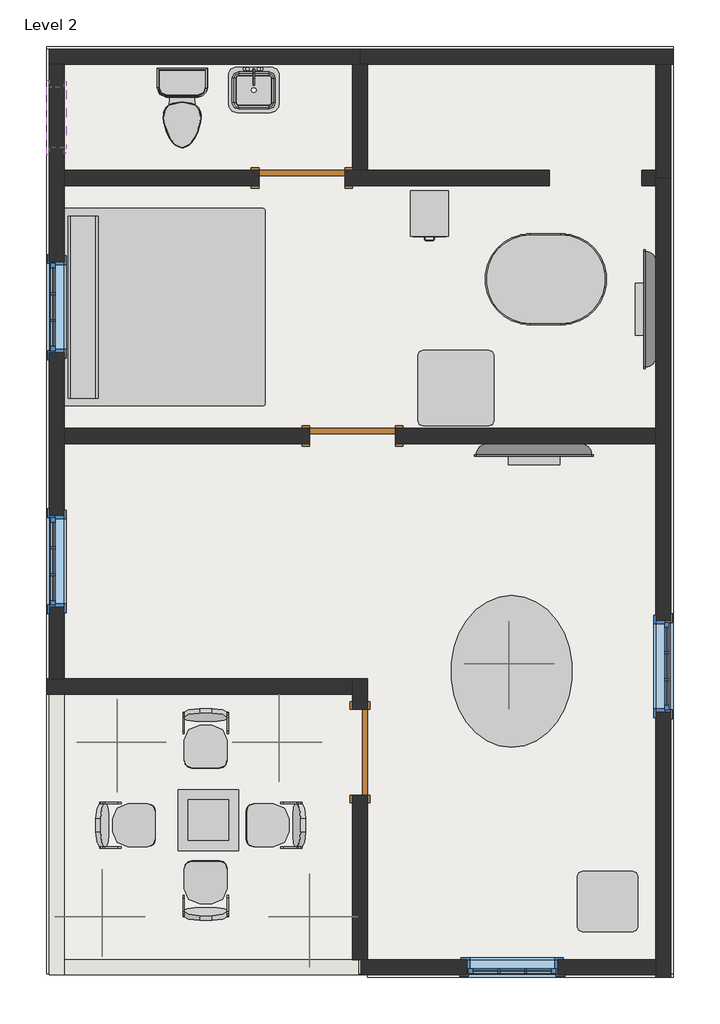
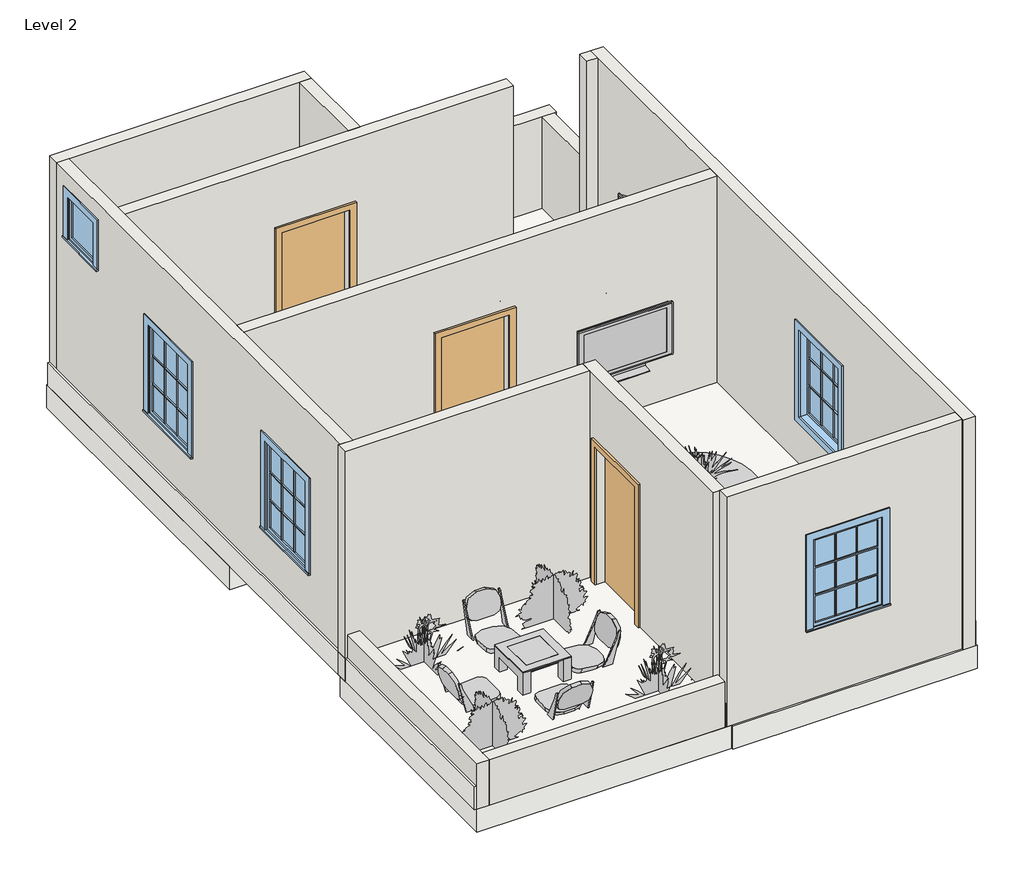
# One storey, incomplete: 14 walls, 13 furniture elements, 5 geographic elements, 5 windows, 4 slabs, 3 doors, 3 flow terminals, 1 roof.
"""IFC4 building model written with IfcOpenShell, lengths in millimetres."""

from ifc_helpers import new_model, si_unit, frame, origin, place, context, project, spatial, polyline, outline, extrude, faceted_brep, transform, mapped, element, save
from components import door_b6e9fca3, door_99d96fc5, flow_terminal_accce45a, flow_terminal_62a433f7, toilet_domestic_3d_toilet_domestic_3d_f7549cf7, toilet_domestic_3d_toilet_domestic_3d_183bbd19, furniture_1fc5af50, furniture_bb55ed6b, furniture_3d1d9cbc, furniture_d9bcc661, furniture_b5c51a22, furniture_be1c6672, furniture_743965d2, furniture_31d08a24, furniture_db92a8cd, rpc_plant_tropical_55f6ff97, rpc_plant_tropical_agave_1_5_93a2a214, rpc_plant_tropical_jungle_flame_3_9c4808c2, window_5c190c7e, window_3d781103

model = new_model("IFC4")

# Units and contexts
model_context = context("Model", 3, world=origin())
ifc_project = project(units=[si_unit("LENGTHUNIT", "METRE", prefix="MILLI")], contexts=[model_context])

# Site, building, storey
site = spatial("IfcSite", under=ifc_project)
building = spatial("IfcBuilding", under=site)
storey = spatial("IfcBuildingStorey", under=building, Name="Level 2", Elevation=3048.0)

# Doors
placement = place(None, origin())
door_shape = door_b6e9fca3(model_context)
element("IfcDoor", 1, ObjectType="Single-Flush : 34\" x 84\"", at=placement, inside=storey, context=model_context, shape_type="MappedRepresentation", body=[
    mapped(door_shape, transform((-14219.4170266, 11794.2465295, 3048.0), x_axis=(1.0, 0.0, 0.0), y_axis=(0.0, 1.0, 0.0), z_axis=(0.0, 0.0, 1.0))),
])
element("IfcDoor", 2, ObjectType="Single-Flush : 34\" x 84\"", at=placement, inside=storey, context=model_context, shape_type="MappedRepresentation", body=[
    mapped(door_shape, transform((-13711.4170266, 9203.4465295, 3048.0), x_axis=(1.0, 0.0, 0.0), y_axis=(0.0, 1.0, 0.0), z_axis=(0.0, 0.0, 1.0))),
])
door_2_shape = door_99d96fc5(model_context)
element("IfcDoor", 3, ObjectType="Single-Flush : 34\" x 84\"", at=placement, inside=storey, context=model_context, shape_type="MappedRepresentation", body=[
    mapped(door_2_shape, transform((-13635.2170266, 6028.4465295, 3048.0), x_axis=(0.0, 1.0, 0.0), y_axis=(-1.0, 0.0, 0.0), z_axis=(0.0, 0.0, 1.0))),
])

# Flow terminals
flow_terminal_shape = flow_terminal_accce45a(model_context)
element("IfcFlowTerminal", 4, ObjectType="Floor Drain - Round : 5\" Strainer - 2\" Drain", at=placement, inside=storey, context=model_context, shape_type="MappedRepresentation", body=[
    mapped(flow_terminal_shape, transform((-16234.7800266, 12603.0079295, 3048.0), x_axis=(1.0, 0.0, 0.0), y_axis=(0.0, 1.0, 0.0), z_axis=(0.0, 0.0, 1.0))),
])
flow_terminal_2_shape = flow_terminal_62a433f7(model_context)
element("IfcFlowTerminal", 5, ObjectType="Sink Vanity-Square : 20\" x 18\"", at=placement, inside=storey, context=model_context, shape_type="MappedRepresentation", body=[
    mapped(flow_terminal_2_shape, transform((-14717.7062671, 12727.6625283, 3048.0), x_axis=(1.0, 0.0, 0.0), y_axis=(0.0, 1.0, 0.0), z_axis=(0.0, 0.0, 1.0))),
])
toilet_domestic_3d_toilet_domestic_3d_shape = toilet_domestic_3d_toilet_domestic_3d_f7549cf7(model_context)
toilet_domestic_3d_toilet_domestic_3d_2_shape = toilet_domestic_3d_toilet_domestic_3d_183bbd19(model_context)
element("IfcFlowTerminal", 6, ObjectType="Toilet-Domestic-3D : Toilet-Domestic-3D", at=placement, inside=storey, context=model_context, shape_type="MappedRepresentation", body=[
    mapped(toilet_domestic_3d_toilet_domestic_3d_shape, transform((-15421.9038266, 12403.8465295, 3048.0), x_axis=(1.0, 0.0, 0.0), y_axis=(0.0, 1.0, 0.0), z_axis=(0.0, 0.0, 1.0))),
    mapped(toilet_domestic_3d_toilet_domestic_3d_2_shape, transform((-15421.9038266, 12403.8465295, 3048.0), x_axis=(1.0, 0.0, 0.0), y_axis=(0.0, 1.0, 0.0), z_axis=(0.0, 0.0, 1.0))),
])

# Furniture
furniture_shape = furniture_1fc5af50(model_context)
element("IfcFurniture", 7, ObjectType="Bed-Standard.0001 : King 78\" x 80\"", at=placement, inside=storey, context=model_context, shape_type="MappedRepresentation", body=[
    mapped(furniture_shape, transform((-15649.3121085, 10227.3580049, 3048.0), x_axis=(0.0, 1.0, 0.0), y_axis=(-1.0, 0.0, 0.0), z_axis=(0.0, 0.0, 1.0))),
])
furniture_2_shape = furniture_bb55ed6b(model_context)
element("IfcFurniture", 8, ObjectType="Cabinet-File 2 Drawer : 15\" x 18\"", at=placement, inside=storey, context=model_context, shape_type="MappedRepresentation", body=[
    mapped(furniture_2_shape, transform((-12808.8205795, 11580.7808296, 3048.0), x_axis=(1.0, 0.0, 0.0), y_axis=(0.0, 1.0, 0.0), z_axis=(0.0, 0.0, 1.0))),
])
furniture_3_shape = furniture_3d1d9cbc(model_context)
element("IfcFurniture", 9, ObjectType="Seating-Auditorium : 18\" x 24\" x 30\"", at=placement, inside=storey, context=model_context, shape_type="MappedRepresentation", body=[
    mapped(furniture_3_shape, transform((-15023.8891577, 6366.5817393, 3048.0), x_axis=(-1.0000000000000004, 0.0, 0.0), y_axis=(0.0, -1.0000000000000004, 0.0), z_axis=(0.0, 0.0, 1.0))),
])
element("IfcFurniture", 10, ObjectType="Seating-Auditorium : 18\" x 24\" x 30\"", at=placement, inside=storey, context=model_context, shape_type="MappedRepresentation", body=[
    mapped(furniture_3_shape, transform((-15345.3448954, 4441.5711196, 3048.0), x_axis=(1.0, 0.0, 0.0), y_axis=(0.0, 1.0, 0.0), z_axis=(0.0, 0.0, 1.0))),
])
element("IfcFurniture", 11, ObjectType="Seating-Auditorium : 18\" x 24\" x 30\"", at=placement, inside=storey, context=model_context, shape_type="MappedRepresentation", body=[
    mapped(furniture_3_shape, transform((-16187.2924364, 5456.7653983, 3048.0), x_axis=(0.0, -1.0000000000000007, 0.0), y_axis=(1.0000000000000007, 0.0, 0.0), z_axis=(0.0, 0.0, 1.0))),
])
element("IfcFurniture", 12, ObjectType="Seating-Auditorium : 18\" x 24\" x 30\"", at=placement, inside=storey, context=model_context, shape_type="MappedRepresentation", body=[
    mapped(furniture_3_shape, transform((-14283.5416167, 5135.3096606, 3048.0), x_axis=(0.0, 1.0000000000000002, 0.0), y_axis=(-1.0000000000000002, 0.0, 0.0), z_axis=(0.0, 0.0, 1.0))),
])
furniture_4_shape = furniture_d9bcc661(model_context)
element("IfcFurniture", 13, ObjectType="TV - Flat Screen : 46\"", at=placement, inside=storey, context=model_context, shape_type="MappedRepresentation", body=[
    mapped(furniture_4_shape, transform((-10715.6056502, 10473.1984681, 3962.4), x_axis=(0.0, -1.0000000000000007, 0.0), y_axis=(1.0000000000000007, 0.0, 0.0), z_axis=(0.0, 0.0, 1.0))),
])
element("IfcFurniture", 14, ObjectType="TV - Flat Screen : 46\"", at=placement, inside=storey, context=model_context, shape_type="MappedRepresentation", body=[
    mapped(furniture_4_shape, transform((-11882.8889124, 9068.7079058, 3962.4), x_axis=(1.0, 0.0, 0.0), y_axis=(0.0, 1.0, 0.0), z_axis=(0.0, 0.0, 1.0))),
])
furniture_5_shape = furniture_b5c51a22(model_context)
element("IfcFurniture", 15, ObjectType="Table-Coffee : 24\" x 24\" x 24\"", at=placement, inside=storey, context=model_context, shape_type="MappedRepresentation", body=[
    mapped(furniture_5_shape, transform((-15177.4827932, 5251.6264517, 3048.0), x_axis=(1.0, 0.0, 0.0), y_axis=(0.0, 1.0, 0.0), z_axis=(0.0, 0.0, 1.0))),
])
furniture_6_shape = furniture_be1c6672(model_context)
element("IfcFurniture", 16, ObjectType="Table-Dining Oval : 36\" x 48\"", at=placement, inside=storey, context=model_context, shape_type="MappedRepresentation", body=[
    mapped(furniture_6_shape, transform((-11366.4973544, 11136.3448901, 3048.0), x_axis=(1.0, 0.0, 0.0), y_axis=(0.0, 1.0, 0.0), z_axis=(0.0, 0.0, 1.0))),
])
furniture_7_shape = furniture_743965d2(model_context)
element("IfcFurniture", 17, ObjectType="Table-Ellipse : 60\" x 48\"", at=placement, inside=storey, context=model_context, shape_type="MappedRepresentation", body=[
    mapped(furniture_7_shape, transform((-12111.2170266, 6841.2465295, 3048.0), x_axis=(0.0, 1.0000000000000002, 0.0), y_axis=(-1.0000000000000002, 0.0, 0.0), z_axis=(0.0, 0.0, 1.0))),
])
furniture_8_shape = furniture_31d08a24(model_context)
element("IfcFurniture", 18, ObjectType="Table-End : 24\" x 24\"", at=placement, inside=storey, context=model_context, shape_type="MappedRepresentation", body=[
    mapped(furniture_8_shape, transform((-11454.5506569, 4377.4465295, 3048.0), x_axis=(1.0, 0.0, 0.0), y_axis=(0.0, 1.0, 0.0), z_axis=(0.0, 0.0, 1.0))),
])
furniture_9_shape = furniture_db92a8cd(model_context)
element("IfcFurniture", 19, ObjectType="Table-End : 30\" x 30\"", at=placement, inside=storey, context=model_context, shape_type="MappedRepresentation", body=[
    mapped(furniture_9_shape, transform((-13054.7506569, 9533.6465295, 3048.0), x_axis=(1.0, 0.0, 0.0), y_axis=(0.0, 1.0, 0.0), z_axis=(0.0, 0.0, 1.0))),
])

# Geographic elements
rpc_plant_tropical_shape = rpc_plant_tropical_55f6ff97(model_context)
element("IfcGeographicElement", 20, ObjectType="RPC Plant - Tropical", at=placement, inside=storey, context=model_context, shape_type="MappedRepresentation", body=[
    mapped(rpc_plant_tropical_shape, transform((-16073.6170266, 6130.0465295, 3048.0), x_axis=(1.0, 0.0, 0.0), y_axis=(0.0, 1.0, 0.0), z_axis=(0.0, 0.0, 1.0))),
])
element("IfcGeographicElement", 21, ObjectType="RPC Plant - Tropical", at=placement, inside=storey, context=model_context, shape_type="MappedRepresentation", body=[
    mapped(rpc_plant_tropical_shape, transform((-14143.2170266, 4377.4465295, 3048.0), x_axis=(1.0, 0.0, 0.0), y_axis=(0.0, 1.0, 0.0), z_axis=(0.0, 0.0, 1.0))),
])
rpc_plant_tropical_agave_1_5_shape = rpc_plant_tropical_agave_1_5_93a2a214(model_context)
element("IfcGeographicElement", 22, ObjectType="RPC Plant - Tropical : Agave - 1.5'", at=placement, inside=storey, context=model_context, shape_type="MappedRepresentation", body=[
    mapped(rpc_plant_tropical_agave_1_5_shape, transform((-12136.6170266, 6917.4465295, 3810.0), x_axis=(1.0, 0.0, 0.0), y_axis=(0.0, 1.0, 0.0), z_axis=(0.0, 0.0, 1.0))),
])
rpc_plant_tropical_jungle_flame_3_shape = rpc_plant_tropical_jungle_flame_3_9c4808c2(model_context)
element("IfcGeographicElement", 23, ObjectType="RPC Plant - Tropical : Jungle Flame - 3'", at=placement, inside=storey, context=model_context, shape_type="MappedRepresentation", body=[
    mapped(rpc_plant_tropical_jungle_flame_3_shape, transform((-16226.0170266, 4377.4465295, 3048.0), x_axis=(1.0, 0.0, 0.0), y_axis=(0.0, 1.0, 0.0), z_axis=(0.0, 0.0, 1.0))),
])
element("IfcGeographicElement", 24, ObjectType="RPC Plant - Tropical : Jungle Flame - 3'", at=placement, inside=storey, context=model_context, shape_type="MappedRepresentation", body=[
    mapped(rpc_plant_tropical_jungle_flame_3_shape, transform((-14448.0170266, 6130.0465295, 3048.0), x_axis=(1.0, 0.0, 0.0), y_axis=(0.0, 1.0, 0.0), z_axis=(0.0, 0.0, 1.0))),
])

# Roof
element("IfcRoof", 25, ObjectType="Generic - 12\"", at=placement, inside=storey, context=model_context, shape_type="SweptSolid", body=[
    extrude(outline(polyline([(-16784.8170266, 13085.6587295), (-10485.6170266, 13085.6587295), (-10485.6170266, 3805.9465295), (-16784.8170266, 3805.9465295), (-16784.8170266, 13085.6587295)])), frame((0.0, 0.0, 3048.0), z_axis=(0.0, 0.0, 1.0), x_axis=(1.0, 0.0, 0.0)), (0.0, 0.0, 1.0), 304.8),
])

# Slabs
element("IfcSlab", 26, ObjectType="Generic - 12\"", at=placement, inside=storey, context=model_context, shape_type="SweptSolid", body=[
    extrude(outline(polyline([(-10485.6170266, 13115.0465295), (-10485.6170266, 9127.2465295), (-16784.8170266, 9127.2465295), (-16784.8170266, 13115.0465295), (-10485.6170266, 13115.0465295)])), frame((0.0, 0.0, 2743.2), z_axis=(0.0, 0.0, 1.0), x_axis=(1.0, 0.0, 0.0)), (0.0, 0.0, 1.0), 304.8),
])
element("IfcSlab", 27, ObjectType="Generic - 12\"", at=placement, inside=storey, context=model_context, shape_type="SweptSolid", body=[
    extrude(outline(polyline([(-13559.0170266, 6765.0465295), (-13559.0170266, 3793.2465295), (-16759.4170266, 3793.2465295), (-16759.4170266, 6765.0465295), (-13559.0170266, 6765.0465295)])), frame((0.0, 0.0, 2743.2), z_axis=(0.0, 0.0, 1.0), x_axis=(1.0, 0.0, 0.0)), (0.0, 0.0, 1.0), 304.8),
])
element("IfcSlab", 28, ObjectType="Generic - 12\"", at=placement, inside=storey, context=model_context, shape_type="SweptSolid", body=[
    extrude(outline(polyline([(-10485.6170266, 9127.2465295), (-10485.6170266, 3767.8465295), (-13559.0170266, 3767.8465295), (-13559.0170266, 9127.2465295), (-10485.6170266, 9127.2465295)])), frame((0.0, 0.0, 2743.2), z_axis=(0.0, 0.0, 1.0), x_axis=(1.0, 0.0, 0.0)), (0.0, 0.0, 1.0), 304.8),
])
element("IfcSlab", 29, ObjectType="Generic - 12\"", at=placement, inside=storey, context=model_context, shape_type="SweptSolid", body=[
    extrude(outline(polyline([(-13559.0170266, 9101.8465295), (-13559.0170266, 6765.0465295), (-14244.8170266, 6765.0465295), (-14244.8170266, 9101.8465295), (-13559.0170266, 9101.8465295)])), frame((0.0, 0.0, 2743.2), z_axis=(0.0, 0.0, 1.0), x_axis=(1.0, 0.0, 0.0)), (0.0, 0.0, 1.0), 304.8),
])

# Walls
element("IfcWall", 30, ObjectType="Generic - 8\"", at=placement, inside=storey, context=model_context, shape_type="Brep", body=[
    faceted_brep([(-16759.4170266, 12937.2465295, 3048.0), (-16607.0170266, 12937.2465295, 3048.0), (-13711.4170266, 12937.2465295, 3048.0), (-13635.2170266, 12937.2465295, 3048.0), (-13635.2170266, 12937.2465295, 4572.0), (-13559.0170266, 12937.2465295, 4572.0), (-13559.0170266, 12937.2465295, 6096.0), (-13711.4170266, 12937.2465295, 6096.0), (-16607.0170266, 12937.2465295, 6096.0), (-16759.4170266, 12937.2465295, 6096.0), (-16759.4170266, 13089.6465295, 3048.0), (-16759.4170266, 13089.6465295, 6096.0), (-13559.0170266, 13089.6465295, 6096.0), (-13559.0170266, 13089.6465295, 4572.0), (-13635.2170266, 13089.6465295, 4572.0), (-13635.2170266, 13089.6465295, 3048.0)], [[[0, 1, 2, 3, 4, 5, 6, 7, 8, 9]], [[10, 11, 12, 13, 14, 15]], [[3, 2, 1, 0, 10, 15]], [[9, 8, 7, 6, 12, 11]], [[0, 9, 11, 10]], [[4, 3, 15, 14]], [[13, 5, 4, 14]], [[6, 5, 13, 12]]]),
])
element("IfcWall", 31, ObjectType="Generic - 8\"", at=placement, inside=storey, context=model_context, shape_type="Brep", body=[
    faceted_brep([(-10663.4170266, 12937.2465295, 3048.0), (-10663.4170266, 11870.4465295, 3048.0), (-10663.4170266, 11794.2465295, 3048.0), (-10663.4170266, 11794.2465295, 4572.0), (-10663.4170266, 11870.4465295, 4572.0), (-10663.4170266, 12937.2465295, 4572.0), (-10511.0170266, 12937.2465295, 3048.0), (-10511.0170266, 12937.2465295, 4572.0), (-10511.0170266, 11870.4465295, 4572.0), (-10511.0170266, 11794.2465295, 4572.0), (-10511.0170266, 11794.2465295, 3048.0)], [[[0, 1, 2, 3, 4, 5]], [[6, 7, 8, 9, 10]], [[2, 1, 0, 6, 10]], [[3, 2, 10, 9]], [[5, 4, 3, 9, 8, 7]], [[0, 5, 7, 6]]]),
])
element("IfcWall", 32, ObjectType="Generic - 8\"", at=placement, inside=storey, context=model_context, shape_type="SweptSolid", body=[
    extrude(outline(polyline([(3048.0, -10663.4170266), (6096.0, -10663.4170266), (6096.0, -13622.5170266), (3048.0, -13622.5170266), (3048.0, -10663.4170266)]), holes=[polyline([(5181.6, -12562.0670266), (5181.6, -11647.6670266), (3962.4, -11647.6670266), (3962.4, -12562.0670266), (5181.6, -12562.0670266)])]), frame((0.0, 3793.2465295, 0.0), z_axis=(0.0, 1.0, 0.0), x_axis=(0.0, 0.0, 1.0)), (0.0, 0.0, 1.0), 152.4),
])
element("IfcWall", 33, ObjectType="Generic - 8\"", at=placement, inside=storey, context=model_context, shape_type="Brep", body=[
    faceted_brep([(-13559.0170266, 6460.2465295, 5181.6), (-13559.0170266, 6460.2465295, 3048.0), (-13559.0170266, 6765.0465295, 3048.0), (-13559.0170266, 6765.0465295, 6096.0), (-13559.0170266, 3945.6465295, 6096.0), (-13559.0170266, 3945.6465295, 3048.0), (-13559.0170266, 5596.6465295, 3048.0), (-13559.0170266, 5596.6465295, 5181.6), (-13711.4170266, 6765.0465295, 3048.0), (-13711.4170266, 6612.6465295, 3048.0), (-13711.4170266, 6460.2465295, 3048.0), (-13711.4170266, 6460.2465295, 5181.6), (-13711.4170266, 5596.6465295, 5181.6), (-13711.4170266, 5596.6465295, 3048.0), (-13711.4170266, 3945.6465295, 3048.0), (-13711.4170266, 3945.6465295, 6096.0), (-13711.4170266, 6612.6465295, 6096.0), (-13711.4170266, 6765.0465295, 6096.0), (-13647.9170266, 3945.6465295, 3048.0)], [[[0, 1, 2, 3, 4, 5, 6, 7]], [[8, 9, 10, 11, 12, 13, 14, 15, 16, 17]], [[6, 5, 18, 14, 13]], [[2, 1, 10, 9, 8]], [[4, 3, 17, 16, 15]], [[5, 4, 15, 14, 18]], [[3, 2, 8, 17]], [[11, 10, 1, 0]], [[12, 11, 0, 7]], [[13, 12, 7, 6]]]),
])
element("IfcWall", 34, ObjectType="Generic - 8\"", at=placement, inside=storey, context=model_context, shape_type="Brep", body=[
    faceted_brep([(-13711.4170266, 6765.0465295, 3048.0), (-16607.0170266, 6765.0465295, 3048.0), (-16759.4170266, 6765.0465295, 3048.0), (-16784.8170266, 6765.0465295, 3048.0), (-16784.8170266, 6765.0465295, 6096.0), (-16759.4170266, 6765.0465295, 6096.0), (-16607.0170266, 6765.0465295, 6096.0), (-13711.4170266, 6765.0465295, 6096.0), (-13711.4170266, 6612.6465295, 3048.0), (-13711.4170266, 6612.6465295, 6096.0), (-16784.8170266, 6612.6465295, 6096.0), (-16784.8170266, 6612.6465295, 3048.0), (-16759.4170266, 6612.6465295, 3048.0), (-16607.0170266, 6612.6465295, 3048.0)], [[[0, 1, 2, 3, 4, 5, 6, 7]], [[8, 9, 10, 11, 12, 13]], [[3, 2, 1, 0, 8, 13, 12, 11]], [[4, 3, 11, 10]], [[7, 6, 5, 4, 10, 9]], [[0, 7, 9, 8]]]),
])
element("IfcWall", 35, ObjectType="Generic - 8\"", at=placement, inside=storey, context=model_context, shape_type="Brep", body=[
    faceted_brep([(-16607.0170266, 6765.0465295, 6096.0), (-16607.0170266, 6765.0465295, 3048.0), (-16607.0170266, 9127.2465295, 3048.0), (-16607.0170266, 9279.6465295, 3048.0), (-16607.0170266, 11718.0465295, 3048.0), (-16607.0170266, 11870.4465295, 3048.0), (-16607.0170266, 12937.2465295, 3048.0), (-16607.0170266, 12937.2465295, 6096.0), (-16607.0170266, 11870.4465295, 6096.0), (-16607.0170266, 11718.0465295, 6096.0), (-16607.0170266, 9279.6465295, 6096.0), (-16607.0170266, 9127.2465295, 6096.0), (-16607.0170266, 12708.6465295, 5816.6), (-16607.0170266, 12708.6465295, 5207.0), (-16607.0170266, 12099.0465295, 5207.0), (-16607.0170266, 12099.0465295, 5816.6), (-16607.0170266, 10956.0465295, 5181.6), (-16607.0170266, 10956.0465295, 3962.4), (-16607.0170266, 10041.6465295, 3962.4), (-16607.0170266, 10041.6465295, 5181.6), (-16607.0170266, 8403.3465295, 5181.6), (-16607.0170266, 8403.3465295, 3962.4), (-16607.0170266, 7488.9465295, 3962.4), (-16607.0170266, 7488.9465295, 5181.6), (-16759.4170266, 6765.0465295, 3048.0), (-16759.4170266, 6765.0465295, 6096.0), (-16759.4170266, 12937.2465295, 6096.0), (-16759.4170266, 12937.2465295, 3048.0), (-16759.4170266, 12708.6465295, 5816.6), (-16759.4170266, 12099.0465295, 5816.6), (-16759.4170266, 12099.0465295, 5207.0), (-16759.4170266, 12708.6465295, 5207.0), (-16759.4170266, 10956.0465295, 5181.6), (-16759.4170266, 10041.6465295, 5181.6), (-16759.4170266, 10041.6465295, 3962.4), (-16759.4170266, 10956.0465295, 3962.4), (-16759.4170266, 8403.3465295, 5181.6), (-16759.4170266, 7488.9465295, 5181.6), (-16759.4170266, 7488.9465295, 3962.4), (-16759.4170266, 8403.3465295, 3962.4)], [[[0, 1, 2, 3, 4, 5, 6, 7, 8, 9, 10, 11], [12, 13, 14, 15], [16, 17, 18, 19], [20, 21, 22, 23]], [[24, 25, 26, 27], [28, 29, 30, 31], [32, 33, 34, 35], [36, 37, 38, 39]], [[6, 5, 4, 3, 2, 1, 24, 27]], [[0, 11, 10, 9, 8, 7, 26, 25]], [[7, 6, 27, 26]], [[13, 12, 28, 31]], [[14, 13, 31, 30]], [[15, 14, 30, 29]], [[12, 15, 29, 28]], [[0, 25, 24, 1]], [[17, 16, 32, 35]], [[18, 17, 35, 34]], [[19, 18, 34, 33]], [[16, 19, 33, 32]], [[21, 20, 36, 39]], [[22, 21, 39, 38]], [[23, 22, 38, 37]], [[20, 23, 37, 36]]]),
])
element("IfcWall", 36, ObjectType="Generic - 8\"", at=placement, inside=storey, context=model_context, shape_type="Brep", body=[
    faceted_brep([(-16759.4170266, 6612.6465295, 3048.0), (-16759.4170266, 3793.2465295, 3048.0), (-16759.4170266, 3793.2465295, 3657.6), (-16759.4170266, 6612.6465295, 3657.6), (-16607.0170266, 6612.6465295, 3048.0), (-16607.0170266, 6612.6465295, 3657.6), (-16607.0170266, 3945.6465295, 3657.6), (-16607.0170266, 3793.2465295, 3657.6), (-16607.0170266, 3793.2465295, 3048.0), (-16607.0170266, 3945.6465295, 3048.0)], [[[0, 1, 2, 3]], [[4, 5, 6, 7, 8, 9]], [[1, 0, 4, 9, 8]], [[3, 2, 7, 6, 5]], [[0, 3, 5, 4]], [[2, 1, 8, 7]]]),
])
element("IfcWall", 37, ObjectType="Generic - 8\"", at=placement, inside=storey, context=model_context, shape_type="Brep", body=[
    faceted_brep([(-13787.6170266, 11718.0465295, 5181.6), (-13787.6170266, 11718.0465295, 3048.0), (-11730.2170266, 11718.0465295, 3048.0), (-11730.2170266, 11718.0465295, 6096.0), (-16607.0170266, 11718.0465295, 6096.0), (-16607.0170266, 11718.0465295, 3048.0), (-14651.2170266, 11718.0465295, 3048.0), (-14651.2170266, 11718.0465295, 5181.6), (-11730.2170266, 11870.4465295, 3048.0), (-13559.0170266, 11870.4465295, 3048.0), (-13711.4170266, 11870.4465295, 3048.0), (-13787.6170266, 11870.4465295, 3048.0), (-13787.6170266, 11870.4465295, 5181.6), (-14651.2170266, 11870.4465295, 5181.6), (-14651.2170266, 11870.4465295, 3048.0), (-16607.0170266, 11870.4465295, 3048.0), (-16607.0170266, 11870.4465295, 6096.0), (-13711.4170266, 11870.4465295, 6096.0), (-13559.0170266, 11870.4465295, 6096.0), (-11730.2170266, 11870.4465295, 6096.0)], [[[0, 1, 2, 3, 4, 5, 6, 7]], [[8, 9, 10, 11, 12, 13, 14, 15, 16, 17, 18, 19]], [[6, 5, 15, 14]], [[2, 1, 11, 10, 9, 8]], [[3, 2, 8, 19]], [[4, 3, 19, 18, 17, 16]], [[5, 4, 16, 15]], [[12, 11, 1, 0]], [[13, 12, 0, 7]], [[14, 13, 7, 6]]]),
])
element("IfcWall", 38, ObjectType="Generic - 8\"", at=placement, inside=storey, context=model_context, shape_type="Brep", body=[
    faceted_brep([(-13559.0170266, 11870.4465295, 3048.0), (-13559.0170266, 12937.2465295, 3048.0), (-13559.0170266, 12937.2465295, 4572.0), (-13559.0170266, 12937.2465295, 6096.0), (-13559.0170266, 11870.4465295, 6096.0), (-13711.4170266, 11870.4465295, 3048.0), (-13711.4170266, 11870.4465295, 6096.0), (-13711.4170266, 12937.2465295, 6096.0), (-13711.4170266, 12937.2465295, 3048.0), (-13635.2170266, 12937.2465295, 3048.0)], [[[0, 1, 2, 3, 4]], [[5, 6, 7, 8]], [[1, 0, 5, 8, 9]], [[4, 3, 7, 6]], [[0, 4, 6, 5]], [[1, 9, 8, 7, 3, 2]]]),
])
element("IfcWall", 39, ObjectType="Generic - 8\"", at=placement, inside=storey, context=model_context, shape_type="SweptSolid", body=[
    extrude(outline(polyline([(5181.6, -13279.6170266), (3048.0, -13279.6170266), (3048.0, -10663.4170266), (6096.0, -10663.4170266), (6096.0, -16607.0170266), (3048.0, -16607.0170266), (3048.0, -14143.2170266), (5181.6, -14143.2170266), (5181.6, -13279.6170266)])), frame((0.0, 9127.2465295, 0.0), z_axis=(0.0, 1.0, 0.0), x_axis=(0.0, 0.0, 1.0)), (0.0, 0.0, 1.0), 152.4),
])
element("IfcWall", 40, ObjectType="Generic - 8\"", at=placement, inside=storey, context=model_context, shape_type="Brep", body=[
    faceted_brep([(-13635.2170266, 12937.2465295, 3048.0), (-13559.0170266, 12937.2465295, 3048.0), (-10663.4170266, 12937.2465295, 3048.0), (-10511.0170266, 12937.2465295, 3048.0), (-10485.6170266, 12937.2465295, 3048.0), (-10485.6170266, 12937.2465295, 4572.0), (-10511.0170266, 12937.2465295, 4572.0), (-10663.4170266, 12937.2465295, 4572.0), (-13559.0170266, 12937.2465295, 4572.0), (-13635.2170266, 12937.2465295, 4572.0), (-13635.2170266, 13089.6465295, 3048.0), (-13635.2170266, 13089.6465295, 4572.0), (-13559.0170266, 13089.6465295, 4572.0), (-10485.6170266, 13089.6465295, 4572.0), (-10485.6170266, 13089.6465295, 3048.0)], [[[0, 1, 2, 3, 4, 5, 6, 7, 8, 9]], [[10, 11, 12, 13, 14]], [[4, 3, 2, 1, 0, 10, 14]], [[5, 4, 14, 13]], [[9, 8, 7, 6, 5, 13, 12, 11]], [[0, 9, 11, 10]]]),
])
element("IfcWall", 41, ObjectType="Generic - 8\"", at=placement, inside=storey, context=model_context, shape_type="Brep", body=[
    faceted_brep([(-10663.4170266, 11794.2465295, 3048.0), (-10663.4170266, 11718.0465295, 3048.0), (-10663.4170266, 9279.6465295, 3048.0), (-10663.4170266, 9127.2465295, 3048.0), (-10663.4170266, 3945.6465295, 3048.0), (-10663.4170266, 3793.2465295, 3048.0), (-10663.4170266, 3767.8465295, 3048.0), (-10663.4170266, 3767.8465295, 6096.0), (-10663.4170266, 3793.2465295, 6096.0), (-10663.4170266, 3945.6465295, 6096.0), (-10663.4170266, 9127.2465295, 6096.0), (-10663.4170266, 9279.6465295, 6096.0), (-10663.4170266, 11718.0465295, 6096.0), (-10663.4170266, 11870.4465295, 6096.0), (-10663.4170266, 11870.4465295, 4572.0), (-10663.4170266, 11794.2465295, 4572.0), (-10663.4170266, 6434.8465295, 5181.6), (-10663.4170266, 6434.8465295, 3962.4), (-10663.4170266, 7349.2465295, 3962.4), (-10663.4170266, 7349.2465295, 5181.6), (-10511.0170266, 11794.2465295, 3048.0), (-10511.0170266, 11794.2465295, 4572.0), (-10511.0170266, 11870.4465295, 4572.0), (-10511.0170266, 11870.4465295, 6096.0), (-10511.0170266, 3767.8465295, 6096.0), (-10511.0170266, 3767.8465295, 3048.0), (-10511.0170266, 6434.8465295, 5181.6), (-10511.0170266, 7349.2465295, 5181.6), (-10511.0170266, 7349.2465295, 3962.4), (-10511.0170266, 6434.8465295, 3962.4)], [[[0, 1, 2, 3, 4, 5, 6, 7, 8, 9, 10, 11, 12, 13, 14, 15], [16, 17, 18, 19]], [[20, 21, 22, 23, 24, 25], [26, 27, 28, 29]], [[6, 5, 4, 3, 2, 1, 0, 20, 25]], [[7, 6, 25, 24]], [[13, 12, 11, 10, 9, 8, 7, 24, 23]], [[0, 15, 21, 20]], [[14, 22, 21, 15]], [[14, 13, 23, 22]], [[17, 16, 26, 29]], [[18, 17, 29, 28]], [[19, 18, 28, 27]], [[16, 19, 27, 26]]]),
])
element("IfcWall", 42, ObjectType="Generic - 8\"", at=placement, inside=storey, context=model_context, shape_type="Brep", body=[
    faceted_brep([(-13647.9170266, 3945.6465295, 3048.0), (-13711.4170266, 3945.6465295, 3048.0), (-16607.0170266, 3945.6465295, 3048.0), (-16607.0170266, 3945.6465295, 3657.6), (-13647.9170266, 3945.6465295, 3657.6), (-13647.9170266, 3793.2465295, 3048.0), (-13647.9170266, 3793.2465295, 3657.6), (-16607.0170266, 3793.2465295, 3657.6), (-16607.0170266, 3793.2465295, 3048.0)], [[[0, 1, 2, 3, 4]], [[5, 6, 7, 8]], [[2, 1, 0, 5, 8]], [[4, 3, 7, 6]], [[0, 4, 6, 5]], [[3, 2, 8, 7]]]),
])
element("IfcWall", 43, ObjectType="Generic - 8\"", at=placement, inside=storey, context=model_context, shape_type="Brep", body=[
    faceted_brep([(-10803.1170266, 11718.0465295, 3048.0), (-10663.4170266, 11718.0465295, 3048.0), (-10663.4170266, 11718.0465295, 6096.0), (-10803.1170266, 11718.0465295, 6096.0), (-10803.1170266, 11870.4465295, 3048.0), (-10803.1170266, 11870.4465295, 6096.0), (-10663.4170266, 11870.4465295, 6096.0), (-10663.4170266, 11870.4465295, 4572.0), (-10663.4170266, 11870.4465295, 3048.0), (-10663.4170266, 11794.2465295, 3048.0)], [[[0, 1, 2, 3]], [[4, 5, 6, 7, 8]], [[1, 0, 4, 8, 9]], [[3, 2, 6, 5]], [[0, 3, 5, 4]], [[1, 9, 8, 7, 6, 2]]]),
])

# Windows
window_shape = window_5c190c7e(model_context)
element("IfcWindow", 44, ObjectType="Casement 3x3 with Trim : 36\" x 48\"", at=placement, inside=storey, context=model_context, shape_type="MappedRepresentation", body=[
    mapped(window_shape, transform((-16683.2170266, 10498.8465295, 3048.0), x_axis=(0.0, 1.0, 0.0), y_axis=(-1.0, 0.0, 0.0), z_axis=(0.0, 0.0, 1.0))),
])
element("IfcWindow", 45, ObjectType="Casement 3x3 with Trim : 36\" x 48\"", at=placement, inside=storey, context=model_context, shape_type="MappedRepresentation", body=[
    mapped(window_shape, transform((-16683.2170266, 7946.1465295, 3048.0), x_axis=(0.0, 1.0, 0.0), y_axis=(-1.0, 0.0, 0.0), z_axis=(0.0, 0.0, 1.0))),
])
element("IfcWindow", 46, ObjectType="Casement 3x3 with Trim : 36\" x 48\"", at=placement, inside=storey, context=model_context, shape_type="MappedRepresentation", body=[
    mapped(window_shape, transform((-12104.8670266, 3869.4465295, 3048.0), x_axis=(-1.0, 0.0, 0.0), y_axis=(0.0, -1.0, 0.0), z_axis=(0.0, 0.0, 1.0))),
])
element("IfcWindow", 47, ObjectType="Casement 3x3 with Trim : 36\" x 48\"", at=placement, inside=storey, context=model_context, shape_type="MappedRepresentation", body=[
    mapped(window_shape, transform((-10587.2170266, 6892.0465295, 3048.0), x_axis=(0.0, -1.0, 0.0), y_axis=(1.0, 0.0, 0.0), z_axis=(0.0, 0.0, 1.0))),
])
window_2_shape = window_3d781103(model_context)
element("IfcWindow", 48, ObjectType="Transom with Trim : 24\" x 24\"", at=placement, inside=storey, context=model_context, shape_type="MappedRepresentation", body=[
    mapped(window_2_shape, transform((-16683.2170266, 12441.9465295, 3048.0), x_axis=(0.0, 1.0, 0.0), y_axis=(-1.0, 0.0, 0.0), z_axis=(0.0, 0.0, 1.0))),
])

save(model, "model.ifc")

# Revit data of these elements
# Type "Single-Flush : 34\" x 84\""
#   Type Mark = "2"
#   Construction Type Id = "MDOOR"
#   Assembly Code = "C1020"
#   Analytic Construction = "Metal"
#   Thickness = 0' - 2"
#   Heat Transfer Coefficient (U) = 0.651978 BTU/(h·ft²·°F)
#   Height = 7' - 0"
#   Trim Projection Ext = 0' - 1"
#   Trim Projection Int = 0' - 1"
#   Trim Width = 0' - 3"
#   Width = 2' - 10"
#   Define Thermal Properties by = 1
#   Door Material = Door - Panel
#   Frame Material = Door - Frame
#   Visual Light Transmittance = 0
#   Solar Heat Gain Coefficient = 0
#   Function = (empty or 0)
#   Wall Closure = (empty or 0)
# Type "Floor Drain - Round : 5\" Strainer - 2\" Drain"
#   WFU = 2
#   Strainer Height = 0' - 3 1/4"
#   Strainer Radius = 0' - 2 1/2"
#   Strainer Diameter = 0' - 5"
#   Radius 6 = 0' - 0 5/8"
#   Radius 5 = 0' - 1 1/4"
#   Radius 4 = 0' - 1 7/8"
#   Radius 2 = 0' - 3.04167"
#   Radius 1 = 0' - 2.02083"
#   Radius 3 = 0' - 2 1/32"
#   Pipe Radius = 1"
#   Pipe Diameter = 2"
#   Height 2 = 0' - 0.725"
#   Height 1 = 0' - 1 13/16"
#   Body Radius = 0' - 4 1/16"
#   Body Height = 0' - 3 5/8"
#   Body Diameter = 0' - 8 1/8"
#   Drain Material = none
#   HWFU = 0
#   Default Elevation = 0
#   CWFU = 0
# Type "Sink Vanity-Square : 20\" x 18\""
#   Assembly Code = "D2010400"
#   Counter Height = 2' - 7"
#   Depth = 1' - 6"
#   Width = 1' - 8"
#   Basin Material = Porcelain, Linen
#   Faucet Material = Steel, Polished
#   Default Elevation = 0
# Type "Toilet-Domestic-3D : Toilet-Domestic-3D"
#   Assembly Code = "D2010110"
#   Toilet - Bowl/Basin Material = Porcelain, Linen
#   Toilet - Seat Material = Laminate, Linen, Matte
#   Default Elevation = 0
# Type "Bed-Standard.0001 : King 78\" x 80\""
#   Assembly Code = "E2020200"
#   Length = 6' - 8"
#   Width = 6' - 6"
#   Leg Material = Steel, Chrome Plated
#   Mattress Material = Linen, White
#   Default Elevation = 0
# Type "Cabinet-File 2 Drawer : 15\" x 18\""
#   Assembly Code = "E2020200"
#   Depth = 1' - 6"
#   Height = 2' - 5"
#   Width = 1' - 3"
#   Cabinet Material = Steel, Paint Finish, Ivory, Glossy
#   Handle Material = Steel, Chrome Plated
#   Default Elevation = 0
# Type "Seating-Auditorium : 18\" x 24\" x 30\""
#   Assembly Code = "E2020200"
#   Seat Material = Linen, Beige
#   Frame Material = Steel, Paint Finish, Dark Gray, Matte
#   Default Elevation = 0
# Type "TV - Flat Screen : 46\""
#   SinAng = 0' - 0.0193"
#   L = 3' - 4.83276"
#   H = 1' - 10.97053"
#   Thickness = 0' - 4.33071"
#   Diagonal = 3' - 10.85039"
#   CosAng = 0' - 0.03431"
#   Stand [instance default] = yes
#   Default Elevation = 0
# Type "Table-Coffee : 24\" x 24\" x 24\""
#   Assembly Code = "E2020200"
#   Height = 2' - 0"
#   Length = 2' - 0"
#   Width = 2' - 0"
#   Top Material = none
#   Frame Material = none
#   Default Elevation = 0
# Type "Table-Dining Oval : 36\" x 48\""
#   Assembly Code = "E2020200"
#   Length = 4' - 0"
#   Width = 3' - 0"
#   Base Material = Steel, Chrome Plated
#   Top Material = Glass - Clear, Grey
#   Default Elevation = 0
#   Description = (empty or 0)
# Type "Table-Ellipse : 60\" x 48\""
#   Assembly Code = "E2020200"
#   Half Width = 2' - 0"
#   Half Length = 2' - 6"
#   Height = 2' - 6"
#   Length = 5' - 0"
#   Width = 4' - 0"
#   Base Material = Birch
#   Top Material = Birch
#   Default Elevation = 0
# Type "Table-End : 24\" x 24\""
#   Assembly Code = "E2020200"
#   Height = 2' - 0"
#   Length = 2' - 0"
#   Width = 2' - 0"
#   Base Material = Birch
#   Top Material = Laminate, Ivory, Matte
#   Default Elevation = 0
# Type "Table-End : 30\" x 30\""
#   Assembly Code = "E2020200"
#   Height = 1' - 6"
#   Length = 2' - 6"
#   Width = 2' - 6"
#   Base Material = Birch
#   Top Material = Laminate, Ivory, Matte
#   Default Elevation = 0
# Type "RPC Plant - Tropical"
#   built-in parameter 1005198 = "{2, 15},{39, RPC-16-FWM5-GM7X-C67P-4000-ST1L-LVER-AU},{1, 0},{1, 0},{2, 13},{1, 8},{5, Color},{1, 0},{1, 0},{3, 0.8},{3, 0.8},{3, 0.8},{1, 8},{7, BBoxMin},{1, 0},{1, 0},{1, 0},{1, 0},{1, 0},{1, 8},{7, BBoxMax},{1, 0},{1, 0},{1, 0},{1, 0},{1, 0},{2, 11},{9, RPCTypeId},{1, 0},{1, 0},{39, RPC-16-FWM5-GM7X-C67P-4000-ST1L-LVER-AU},{1, 6},{14, RPCPlantHeight},{1, 0},{1, 0},{1, 3},{2, 11},{7, keyword},{1, 0},{1, 0},{35, :RPCs:Shrubs [General]:Geometry:RPC},{2, 11},{8, category},{1, 0},{1, 0},{16, Shrubs [General]},{2, 11},{12, LocalizedUID},{1, 0},{1, 0},{10, Crane Lily},{2, 14},{6, Height},{1, 0},{1, 0},{1, 3},{1, 2},{16, Cast Reflections},{1, 0},{1, 0},{1, 0},{1, 2},{12, Cast Shadows},{1, 0},{1, 0},{1, 1},{1, 2},{9, Lock View},{1, 0},{1, 0},{1, 0},{1, 4},{5, ViewC},{1, 0},{1, 0},{1, 0},{21, assetlibrary_base.fbx},{1, 5},"
#   built-in parameter 1005195 = "RPC-16-FWM5-GM7X-C67P-4000-ST1L-LVER-AU"
#   Assembly Code = "G2050500"
#   Height = 3' - 0"
#   Default Elevation = 0
# Type "RPC Plant - Tropical : Agave - 1.5'"
#   built-in parameter 1005198 = "{2, 15},{39, RPC-16-G1GJ-63FX-7K5P-N000-ST1L-LVER-AU},{1, 0},{1, 0},{2, 13},{1, 8},{5, Color},{1, 0},{1, 0},{3, 0.8},{3, 0.8},{3, 0.8},{1, 8},{7, BBoxMin},{1, 0},{1, 0},{1, 0},{1, 0},{1, 0},{1, 8},{7, BBoxMax},{1, 0},{1, 0},{1, 0},{1, 0},{1, 0},{2, 11},{9, RPCTypeId},{1, 0},{1, 0},{39, RPC-16-G1GJ-63FX-7K5P-N000-ST1L-LVER-AU},{1, 6},{14, RPCPlantHeight},{1, 0},{1, 0},{3, 1.5},{2, 11},{7, keyword},{1, 0},{1, 0},{35, :RPCs:Plants [General]:Geometry:RPC},{2, 11},{8, category},{1, 0},{1, 0},{16, Plants [General]},{2, 11},{12, LocalizedUID},{1, 0},{1, 0},{5, Agave},{2, 14},{6, Height},{1, 0},{1, 0},{3, 1.5},{1, 2},{16, Cast Reflections},{1, 0},{1, 0},{1, 0},{1, 2},{12, Cast Shadows},{1, 0},{1, 0},{1, 1},{1, 2},{9, Lock View},{1, 0},{1, 0},{1, 0},{1, 4},{5, ViewC},{1, 0},{1, 0},{1, 0},{21, assetlibrary_base.fbx},{1, 5},"
#   built-in parameter 1005195 = "RPC-16-G1GJ-63FX-7K5P-N000-ST1L-LVER-AU"
#   Type Comments = "Agave"
#   Assembly Code = "G2050500"
#   Height = 1' - 6"
#   Default Elevation = 0
# Type "RPC Plant - Tropical : Jungle Flame - 3'"
#   built-in parameter 1005198 = "{2, 15},{39, RPC-16-FUVJ-JWG0-MWGK-8000-ST1L-LVER-AU},{1, 0},{1, 0},{2, 13},{1, 8},{5, Color},{1, 0},{1, 0},{3, 0.8},{3, 0.8},{3, 0.8},{1, 8},{7, BBoxMin},{1, 0},{1, 0},{1, 0},{1, 0},{1, 0},{1, 8},{7, BBoxMax},{1, 0},{1, 0},{1, 0},{1, 0},{1, 0},{2, 11},{9, RPCTypeId},{1, 0},{1, 0},{39, RPC-16-FUVJ-JWG0-MWGK-8000-ST1L-LVER-AU},{1, 6},{14, RPCPlantHeight},{1, 0},{1, 0},{1, 3},{2, 11},{7, keyword},{1, 0},{1, 0},{35, :RPCs:Shrubs [General]:Geometry:RPC},{2, 11},{8, category},{1, 0},{1, 0},{16, Shrubs [General]},{2, 11},{12, LocalizedUID},{1, 0},{1, 0},{12, Jungle Flame},{2, 14},{6, Height},{1, 0},{1, 0},{1, 3},{1, 2},{16, Cast Reflections},{1, 0},{1, 0},{1, 0},{1, 2},{12, Cast Shadows},{1, 0},{1, 0},{1, 1},{1, 2},{9, Lock View},{1, 0},{1, 0},{1, 0},{1, 4},{5, ViewC},{1, 0},{1, 0},{1, 0},{21, assetlibrary_base.fbx},{1, 5},"
#   built-in parameter 1005195 = "RPC-16-FUVJ-JWG0-MWGK-8000-ST1L-LVER-AU"
#   Type Comments = "Jungle Flame"
#   Assembly Code = "G2050500"
#   Height = 3' - 0"
#   Default Elevation = 0
# Type "Generic - 12\""
#   Assembly Code = "B1020"
#   Layers, outside or top first: 1' - 0" "Brick, Common" (function 1)
# Type "Generic - 12\""
#   Assembly Code = "B1010"
#   Function = 0
#   Layers, outside or top first: 1' - 0" "Brick, Common" (function 1)
# Type "Generic - 8\""
#   Assembly Code = "B2010"
#   Layers, outside or top first: 0' - 6" "Brick, Common" (function 1)
# Type "Casement 3x3 with Trim : 36\" x 48\""
#   Type Mark = "10"
#   Construction Type Id = "GSP4R"
#   Assembly Code = "B2020100"
#   Analytic Construction = "1/8 in Pilkington single glazing"
#   Visual Light Transmittance = 0.9
#   Solar Heat Gain Coefficient = 0.78
#   Heat Transfer Coefficient (U) = 0.6496 BTU/(h·ft²·°F)
#   Height = 4' - 0"
#   Default Sill Height = 3' - 0"
#   Trim Projection - Ext. = 0' - 0 1/2"
#   Trim Projection - Int. = 0' - 0 3/4"
#   Trim Width - Exterior = 0' - 3 1/2"
#   Trim Width - Interior = 0' - 3 1/2"
#   Width = 3' - 0"
#   Window Inset = 0' - 0 3/4"
#   Define Thermal Properties by = 1
#   Glass Pane Material = Glass
#   Sash Material = Sash
#   Trim Exterior Material = Trim
#   Trim Interior Material = Trim
#   Wall Closure = (empty or 0)
# Type "Transom with Trim : 24\" x 24\""
#   Type Mark = "13"
#   Construction Type Id = "GSP4R"
#   Assembly Code = "B2020100"
#   Analytic Construction = "1/8 in Pilkington single glazing"
#   Visual Light Transmittance = 0.9
#   Solar Heat Gain Coefficient = 0.78
#   Heat Transfer Coefficient (U) = 0.6496 BTU/(h·ft²·°F)
#   Height = 2' - 0"
#   Default Sill Height = 7' - 1"
#   Trim Projection - Ext. = 0' - 0 1/2"
#   Trim Projection - Int. = 0' - 0 3/4"
#   Trim Width - Exterior = 0' - 3 1/2"
#   Trim Width - Interior = 0' - 3 1/2"
#   Width = 2' - 0"
#   Window Inset = 0' - 0 3/4"
#   Define Thermal Properties by = 1
#   Glass Pane Material = Glass
#   Sash Material = Sash
#   Trim Exterior Material = Trim
#   Trim Interior Material = Trim
#   Wall Closure = (empty or 0)
# Elements 1, 2, 3 (IfcDoor, "Single-Flush : 34\" x 84\"")
#   Phase Created = New Construction
#   Materials on its faces: "Door - Frame", "Door - Panel"
# Element 4 (IfcFlowTerminal, "Floor Drain - Round : 5\" Strainer - 2\" Drain")
#   Mark = "6"
#   Phase Created = New Construction
# Element 5 (IfcFlowTerminal, "Sink Vanity-Square : 20\" x 18\"")
#   Mark = "4"
#   Phase Created = New Construction
#   Materials on its faces: "Porcelain, Linen", "Steel, Polished"
# Element 6 (IfcFlowTerminal, "Toilet-Domestic-3D : Toilet-Domestic-3D")
#   Mark = "5"
#   Phase Created = New Construction
#   Materials on its faces: "Porcelain, Linen", "Laminate, Linen, Matte"
# Element 7 (IfcFurniture, "Bed-Standard.0001 : King 78\" x 80\"")
#   Phase Created = New Construction
#   Materials on its faces: "Linen, White", "Steel, Chrome Plated"
# Element 8 (IfcFurniture, "Cabinet-File 2 Drawer : 15\" x 18\"")
#   Phase Created = New Construction
#   Materials on its faces: "Steel, Chrome Plated", "Steel, Paint Finish, Ivory, Glossy"
# Elements 9, 10, 11, 12 (IfcFurniture, "Seating-Auditorium : 18\" x 24\" x 30\"")
#   Phase Created = New Construction
#   Materials on its faces: "Steel, Paint Finish, Dark Gray, Matte", "Linen, Beige"
# Elements 13, 14 (IfcFurniture, "TV - Flat Screen : 46\"")
#   Stand = yes
#   Phase Created = New Construction
#   Materials on its faces: "TV - Black", "TV - Glass", "TV - Screen"
# Element 15 (IfcFurniture, "Table-Coffee : 24\" x 24\" x 24\"")
#   Phase Created = New Construction
#   Materials on its faces: "Glass - Clear, Grey"
# Element 16 (IfcFurniture, "Table-Dining Oval : 36\" x 48\"")
#   Phase Created = New Construction
#   Materials on its faces: "Steel, Chrome Plated", "Glass - Clear, Grey"
# Element 17 (IfcFurniture, "Table-Ellipse : 60\" x 48\"")
#   Phase Created = New Construction
#   Materials on its faces: "Birch"
# Element 18 (IfcFurniture, "Table-End : 24\" x 24\"")
#   Phase Created = New Construction
#   Materials on its faces: "Laminate, Ivory, Matte", "Birch"
# Element 19 (IfcFurniture, "Table-End : 30\" x 30\"")
#   Phase Created = New Construction
#   Materials on its faces: "Laminate, Ivory, Matte", "Birch"
# Elements 20, 21 (IfcGeographicElement, "RPC Plant - Tropical")
#   Phase Created = New Construction
# Element 22 (IfcGeographicElement, "RPC Plant - Tropical : Agave - 1.5'")
#   Phase Created = New Construction
# Elements 23, 24 (IfcGeographicElement, "RPC Plant - Tropical : Jungle Flame - 3'")
#   Phase Created = New Construction
# Element 25 (IfcRoof, "Generic - 12\"")
#   built-in parameter 1001705 = 11 (stored number, unit not read)
#   built-in parameter 1001710 = 33615
#   Phase Created = New Construction
#   Materials on its faces: "Brick, Common"
# Elements 26, 27, 28, 29 (IfcSlab, "Generic - 12\"")
#   Height Offset From Level = 0' - 0"
#   Phase Created = New Construction
#   Materials on its faces: "Brick, Common"
# Elements 30, 32, 33, 34, 35, 37, 38, 39, 41, 43 (IfcWall, "Generic - 8\"")
#   Top Offset = 0' - 0"
#   Base Offset = 0' - 0"
#   Unconnected Height = 10' - 0"
#   wall height = 10' - 0"
#   Phase Created = New Construction
#   Base Constraint = Level 2
#   Materials on its faces: "Brick, Common"
# Elements 31, 40 (IfcWall, "Generic - 8\"")
#   Top Offset = 0' - 0"
#   Base Offset = 0' - 0"
#   Unconnected Height = 5' - 0"
#   wall height = 5' - 0"
#   Phase Created = New Construction
#   Base Constraint = Level 2
#   Materials on its faces: "Brick, Common"
# Elements 36, 42 (IfcWall, "Generic - 8\"")
#   Top Offset = 0' - 0"
#   Base Offset = 0' - 0"
#   Unconnected Height = 2' - 0"
#   wall height = 2' - 0"
#   Phase Created = New Construction
#   Base Constraint = Level 2
#   Materials on its faces: "Brick, Common"
# Element 44 (IfcWindow, "Casement 3x3 with Trim : 36\" x 48\"")
#   Mark = "7"
#   Phase Created = New Construction
#   Materials on its faces: "Sash", "Glass", "Trim"
# Element 45 (IfcWindow, "Casement 3x3 with Trim : 36\" x 48\"")
#   Mark = "8"
#   Phase Created = New Construction
#   Materials on its faces: "Sash", "Glass", "Trim"
# Element 46 (IfcWindow, "Casement 3x3 with Trim : 36\" x 48\"")
#   Mark = "9"
#   Phase Created = New Construction
#   Materials on its faces: "Sash", "Glass", "Trim"
# Element 47 (IfcWindow, "Casement 3x3 with Trim : 36\" x 48\"")
#   Mark = "10"
#   Phase Created = New Construction
#   Materials on its faces: "Sash", "Glass", "Trim"
# Element 48 (IfcWindow, "Transom with Trim : 24\" x 24\"")
#   Mark = "6"
#   Phase Created = New Construction
#   Materials on its faces: "Sash", "Trim", "Glass"
# Materials
#   "Door - Panel": class "Wood", colour RGB 210 159 95, transparency 0
#   "Door - Frame": colour RGB 118 70 51, transparency 0
#   "Porcelain, Linen": class "Ceramic", colour RGB 249 239 230, transparency 0, Description = "Porcelain, linen", Cost = 0
#   "Steel, Polished": class "Metal", colour RGB 57 57 57, transparency 0, Description = "Polished steel", Cost = 0
#   "Laminate, Linen, Matte": class "Plastic", colour RGB 249 239 230, transparency 0, Description = "Plastic Laminate - Linen, Matte", Cost = 0
#   "Steel, Chrome Plated": class "Metal", colour RGB 17 17 17, transparency 0, Description = "Chromiuim plated steel", Cost = 0
#   "Linen, White": class "Textile", colour RGB 247 247 239, transparency 0, Description = "Linen, white", Cost = 0
#   "Steel, Paint Finish, Ivory, Glossy": class "Metal", colour RGB 247 247 239, transparency 0, Description = "Steel, paint finish, ivory, glossy", Cost = 0
#   "Linen, Beige": class "Textile", colour RGB 249 239 230, transparency 0, Description = "Linen, beige", Cost = 0
#   "Steel, Paint Finish, Dark Gray, Matte": class "Metal", colour RGB 0 0 0, transparency 0, Description = "Steel, paint finish, dark gray, matte", Cost = 0
#   "Glass - Clear, Grey": class "Glass", colour RGB 252 255 255, transparency 0.64
#   "Birch": class "Wood", colour RGB 224 178 126, transparency 0, Description = "Betula Alleghaniensis", Cost = 0
#   "Laminate, Ivory, Matte": class "Plastic", colour RGB 247 247 239, transparency 0, Description = "Plastic Laminate - Ivory, Matte", Cost = 0
#   "Brick, Common": class "Masonry", colour RGB 170 98 104, transparency 0, Description = "Common brick", Cost = 0
#   "Glass": class "Glass", colour RGB 0 128 192, transparency 0.75, Description = "Soda Lime Glass", Cost = 0
#   "Sash": class "Wood", colour RGB 224 178 126, transparency 0
#   "Trim": class "Wood", colour RGB 224 178 126, transparency 0
#   "TV - Black": colour RGB 49 49 49, transparency 0
#   "TV - Glass": colour RGB 157 157 157, transparency 0.9
#   "TV - Screen": colour RGB 0 0 0, transparency 0
# Room at (-15287.422, 12191.97) mm, phase "New Construction", upper level "Level 2", upper offset 10' - 0", lower offset 0' - 0"
#   Number = "6"
#   Name = "TOILET"
# Room at (-11996.715, 12191.97) mm, phase "New Construction", upper level "Level 2", upper offset 10' - 0", lower offset 0' - 0"
#   Number = "7"
